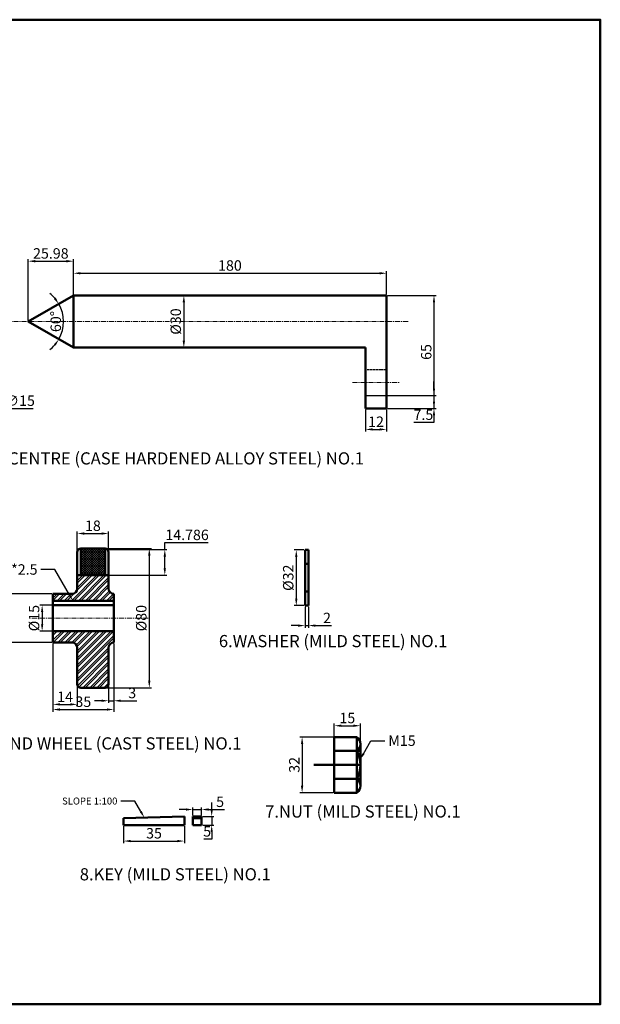
# Model space of a CAD drawing. Units: millimetres. Extents: x 177 to 1064, y 105 to 671.
# Tile 4 of 4: x 730 to 1064, y 105 to 671. Entities that reach past the tile are written whole.
import ezdxf
from ezdxf import colors
from ezdxf.entities.mleader import LeaderData, LeaderLine
from ezdxf.math import Vec2, Vec3

# ---------------------------------------------------------------- set-up
doc = ezdxf.new("R2010")
doc.units = ezdxf.units.MM
doc.header["$LTSCALE"] = 0.3
doc.linetypes.add('CENTER', pattern=[50.8, 31.75, -6.35, 6.35, -6.35])
doc.linetypes.add('HIDDEN', pattern=[9.525, 6.35, -3.175])
for name, color, linetype, lineweight in [('M-CNTR', 1, 'CENTER', 18), ('M-DIMS', 2, 'Continuous', 25), ('M-HATC', 8, 'Continuous', 18), ('M-HIDN', 6, 'HIDDEN', 25), ('M-OUTL', 7, 'Continuous', 50), ('M-TEXT', 3, 'Continuous', 25)]:
    doc.layers.add(name, color=color, linetype=linetype, lineweight=lineweight)
doc.styles.get("Standard").update_dxf_attribs({"font": 'arial.ttf'})
doc.dimstyles.new('ISO-25', dxfattribs={"dimtxt": 6, "dimasz": 4, "dimexe": 1.25, "dimexo": 0.625, "dimtad": 1, "dimtoh": 1, "dimtxsty": 'Standard', "dimcen": 2.5, "dimadec": 0, "dimazin": 0, "dimtfac": 1, "dimtmove": 0, "dimatfit": 3, "dimfxl": 1, "dimarcsym": 0})

# ---------------------------------------------------------------- blocks, each defined once
blk = doc.blocks.new('*D20')
at = {"layer": 'Defpoints', "color": 0, "ltscale": 0.3, "transparency": 16777216}
for p in [(940.65, 525.41), (760.65, 512.65), (940.65, 512.65)]:
    blk.add_point(p, dxfattribs=at)
at = {"layer": 'M-DIMS', "color": 0, "lineweight": -2, "ltscale": 0.3, "transparency": 16777216}
for p, q in [((760.65, 513.28), (760.65, 526.66)), ((940.65, 513.28), (940.65, 526.66)), ((764.65, 525.41), (936.65, 525.41))]:
    blk.add_line(p, q, dxfattribs=at)
at = {"layer": 'M-DIMS', "color": 0, "ltscale": 0.3, "transparency": 16777216}
for points in [[(764.65, 526.08), (764.65, 524.75), (760.65, 525.41)], [(936.65, 526.08), (936.65, 524.75), (940.65, 525.41)]]:
    blk.add_solid(points, dxfattribs=at)
at = {"layer": 'M-DIMS', "color": 0, "ltscale": 0.3, "transparency": 16777216, "insert": (850.65, 529.1), "char_height": 6, "attachment_point": 5}
blk.add_mtext('180', dxfattribs=at)
blk = doc.blocks.new('*D21')
at = {"layer": 'Defpoints', "color": 0, "ltscale": 0.3, "transparency": 16777216}
for p in [(821.8, 512.65), (821.8, 482.65), (824.15, 482.65)]:
    blk.add_point(p, dxfattribs=at)
at = {"layer": 'M-DIMS', "color": 0, "lineweight": -2, "ltscale": 0.3, "transparency": 16777216}
for p, q in [((822.42, 512.65), (825.4, 512.65)), ((824.15, 508.65), (824.15, 486.65)), ((822.42, 482.65), (825.4, 482.65))]:
    blk.add_line(p, q, dxfattribs=at)
at = {"layer": 'M-DIMS', "color": 0, "ltscale": 0.3, "transparency": 16777216}
for points in [[(823.48, 508.65), (824.82, 508.65), (824.15, 512.65)], [(823.48, 486.65), (824.82, 486.65), (824.15, 482.65)]]:
    blk.add_solid(points, dxfattribs=at)
at = {"layer": 'M-DIMS', "color": 0, "ltscale": 0.3, "transparency": 16777216, "insert": (820.29, 497.65), "char_height": 6, "attachment_point": 5, "rotation": 90}
blk.add_mtext('%%C30', dxfattribs=at)
blk = doc.blocks.new('*D22')
at = {"layer": 'Defpoints', "color": 0, "ltscale": 0.3, "transparency": 16777216}
for p in [(928.65, 447.65), (940.65, 447.65), (940.65, 435.63)]:
    blk.add_point(p, dxfattribs=at)
at = {"layer": 'M-DIMS', "color": 0, "lineweight": -2, "ltscale": 0.3, "transparency": 16777216}
for p, q in [((928.65, 447.03), (928.65, 434.38)), ((940.65, 447.03), (940.65, 434.38)), ((932.65, 435.63), (936.65, 435.63))]:
    blk.add_line(p, q, dxfattribs=at)
at = {"layer": 'M-DIMS', "color": 0, "ltscale": 0.3, "transparency": 16777216}
for points in [[(932.65, 436.3), (932.65, 434.97), (928.65, 435.63)], [(936.65, 436.3), (936.65, 434.97), (940.65, 435.63)]]:
    blk.add_solid(points, dxfattribs=at)
at = {"layer": 'M-DIMS', "color": 0, "ltscale": 0.3, "transparency": 16777216, "insert": (934.65, 439.27), "char_height": 6, "attachment_point": 5}
blk.add_mtext('12', dxfattribs=at)
blk = doc.blocks.new('*D25')
at = {"layer": 'Defpoints', "color": 0, "ltscale": 0.3, "transparency": 16777216}
for p in [(696.18, 467.24), (708.04, 458.06)]:
    blk.add_point(p, dxfattribs=at)
at = {"layer": 'M-DIMS', "color": 0, "lineweight": -2, "ltscale": 0.3, "transparency": 16777216}
for p, q in [((693.02, 469.69), (689.85, 472.14)), ((696.18, 467.24), (708.04, 458.06)), ((721.67, 447.51), (711.2, 455.61)), ((737.46, 447.51), (721.67, 447.51))]:
    blk.add_line(p, q, dxfattribs=at)
at = {"layer": 'M-DIMS', "color": 0, "ltscale": 0.3, "transparency": 16777216}
for points in [[(693.43, 470.22), (692.61, 469.16), (696.18, 467.24)], [(711.61, 456.14), (710.8, 455.08), (708.04, 458.06)]]:
    blk.add_solid(points, dxfattribs=at)
at = {"layer": 'M-DIMS', "color": 0, "ltscale": 0.3, "transparency": 16777216, "insert": (729.88, 451.37), "char_height": 6, "attachment_point": 5}
blk.add_mtext('∅15', dxfattribs=at)
blk = doc.blocks.new('*D26')
at = {"layer": 'Defpoints', "color": 0, "ltscale": 0.3, "transparency": 16777216}
for p in [(760.65, 512.65), (734.67, 497.65), (734.67, 497.65), (754.67, 494.12), (760.65, 482.65)]:
    blk.add_point(p, dxfattribs=at)
at = {"layer": 'M-DIMS', "color": 0, "lineweight": -2, "ltscale": 0.3, "transparency": 16777216}
for start, end in [(41.3018, 52.6036), (330, 30), (307.3964, 318.6982)]:
    blk.add_arc((734.67, 497.65), 20.31, start, end, dxfattribs=at)
at = {"layer": 'M-DIMS', "color": 0, "ltscale": 0.3, "transparency": 16777216}
for points in [[(750.47, 511.45), (749.39, 510.67), (752.26, 507.81)], [(749.39, 484.63), (750.47, 483.86), (752.26, 487.49)]]:
    blk.add_solid(points, dxfattribs=at)
at = {"layer": 'M-DIMS', "color": 0, "ltscale": 0.3, "transparency": 16777216, "insert": (751.29, 497.65), "char_height": 6, "attachment_point": 5, "rotation": 90}
blk.add_mtext('60°', dxfattribs=at)
blk = doc.blocks.new('*D27')
at = {"layer": 'Defpoints', "color": 0, "ltscale": 0.3, "transparency": 16777216}
for p in [(773.7, 367.13), (771.87, 287.13), (804.29, 287.13)]:
    blk.add_point(p, dxfattribs=at)
at = {"layer": 'M-DIMS', "color": 0, "lineweight": -2, "ltscale": 0.3, "transparency": 16777216}
for p, q in [((774.32, 367.13), (805.54, 367.13)), ((804.29, 363.13), (804.29, 291.13)), ((772.49, 287.13), (805.54, 287.13))]:
    blk.add_line(p, q, dxfattribs=at)
at = {"layer": 'M-DIMS', "color": 0, "ltscale": 0.3, "transparency": 16777216}
for points in [[(803.62, 363.13), (804.95, 363.13), (804.29, 367.13)], [(803.62, 291.13), (804.95, 291.13), (804.29, 287.13)]]:
    blk.add_solid(points, dxfattribs=at)
at = {"layer": 'M-DIMS', "color": 0, "ltscale": 0.3, "transparency": 16777216, "insert": (800.43, 327.13), "char_height": 6, "attachment_point": 5, "rotation": 90}
blk.add_mtext('%%C80', dxfattribs=at)
blk = doc.blocks.new('*D28')
at = {"layer": 'Defpoints', "color": 0, "ltscale": 0.3, "transparency": 16777216}
for p in [(780.87, 375.78), (762.87, 365.13), (780.87, 365.13)]:
    blk.add_point(p, dxfattribs=at)
at = {"layer": 'M-DIMS', "color": 0, "lineweight": -2, "ltscale": 0.3, "transparency": 16777216}
for p, q in [((762.87, 365.76), (762.87, 377.03)), ((766.87, 375.78), (776.87, 375.78)), ((780.87, 365.76), (780.87, 377.03))]:
    blk.add_line(p, q, dxfattribs=at)
at = {"layer": 'M-DIMS', "color": 0, "ltscale": 0.3, "transparency": 16777216}
for points in [[(766.87, 376.44), (766.87, 375.11), (762.87, 375.78)], [(776.87, 376.44), (776.87, 375.11), (780.87, 375.78)]]:
    blk.add_solid(points, dxfattribs=at)
at = {"layer": 'M-DIMS', "color": 0, "ltscale": 0.3, "transparency": 16777216, "insert": (771.87, 379.46), "char_height": 6, "attachment_point": 5}
blk.add_mtext('18', dxfattribs=at)
blk = doc.blocks.new('*D29')
at = {"layer": 'Defpoints', "color": 0, "ltscale": 0.3, "transparency": 16777216}
for p in [(748.87, 341.13), (720.48, 313.13), (748.87, 313.13)]:
    blk.add_point(p, dxfattribs=at)
at = {"layer": 'M-DIMS', "color": 0, "lineweight": -2, "ltscale": 0.3, "transparency": 16777216}
for p, q in [((748.24, 341.13), (719.23, 341.13)), ((720.48, 337.13), (720.48, 317.13)), ((748.24, 313.13), (719.23, 313.13))]:
    blk.add_line(p, q, dxfattribs=at)
at = {"layer": 'M-DIMS', "color": 0, "ltscale": 0.3, "transparency": 16777216}
for points in [[(719.81, 337.13), (721.14, 337.13), (720.48, 341.13)], [(719.81, 317.13), (721.14, 317.13), (720.48, 313.13)]]:
    blk.add_solid(points, dxfattribs=at)
at = {"layer": 'M-DIMS', "color": 0, "ltscale": 0.3, "transparency": 16777216, "insert": (716.62, 327.13), "char_height": 6, "attachment_point": 5, "rotation": 90}
blk.add_mtext('%%C28', dxfattribs=at)
blk = doc.blocks.new('*D30')
at = {"layer": 'Defpoints', "color": 0, "ltscale": 0.3, "transparency": 16777216}
for p in [(756.31, 334.63), (742.67, 319.63), (756.31, 319.63)]:
    blk.add_point(p, dxfattribs=at)
at = {"layer": 'M-DIMS', "color": 0, "lineweight": -2, "ltscale": 0.3, "transparency": 16777216}
for p, q in [((755.68, 334.63), (741.42, 334.63)), ((742.67, 330.63), (742.67, 323.63)), ((755.68, 319.63), (741.42, 319.63))]:
    blk.add_line(p, q, dxfattribs=at)
at = {"layer": 'M-DIMS', "color": 0, "ltscale": 0.3, "transparency": 16777216}
for points in [[(742.01, 330.63), (743.34, 330.63), (742.67, 334.63)], [(742.01, 323.63), (743.34, 323.63), (742.67, 319.63)]]:
    blk.add_solid(points, dxfattribs=at)
at = {"layer": 'M-DIMS', "color": 0, "ltscale": 0.3, "transparency": 16777216, "insert": (738.82, 327.13), "char_height": 6, "attachment_point": 5, "rotation": 90}
blk.add_mtext('%%C15', dxfattribs=at)
blk = doc.blocks.new('*D31')
at = {"layer": 'Defpoints', "color": 0, "ltscale": 0.3, "transparency": 16777216}
for p in [(748.87, 313.13), (783.87, 313.13), (783.87, 274.59)]:
    blk.add_point(p, dxfattribs=at)
at = {"layer": 'M-DIMS', "color": 0, "lineweight": -2, "ltscale": 0.3, "transparency": 16777216}
for p, q in [((748.87, 312.51), (748.87, 273.34)), ((783.87, 312.51), (783.87, 273.34)), ((752.87, 274.59), (779.87, 274.59))]:
    blk.add_line(p, q, dxfattribs=at)
at = {"layer": 'M-DIMS', "color": 0, "ltscale": 0.3, "transparency": 16777216}
for points in [[(752.87, 275.26), (752.87, 273.92), (748.87, 274.59)], [(779.87, 275.26), (779.87, 273.92), (783.87, 274.59)]]:
    blk.add_solid(points, dxfattribs=at)
at = {"layer": 'M-DIMS', "color": 0, "ltscale": 0.3, "transparency": 16777216, "insert": (766.37, 278.28), "char_height": 6, "attachment_point": 5}
blk.add_mtext('35', dxfattribs=at)
blk = doc.blocks.new('*D32')
at = {"layer": 'Defpoints', "color": 0, "ltscale": 0.3, "transparency": 16777216}
for p in [(780.87, 291.61), (783.87, 291.61), (783.87, 279.64)]:
    blk.add_point(p, dxfattribs=at)
at = {"layer": 'M-DIMS', "color": 0, "lineweight": -2, "ltscale": 0.3, "transparency": 16777216}
for p, q in [((780.87, 290.99), (780.87, 278.39)), ((783.87, 290.99), (783.87, 278.39)), ((776.87, 279.64), (772.87, 279.64)), ((780.87, 279.64), (783.87, 279.64)), ((787.87, 279.64), (797.05, 279.64))]:
    blk.add_line(p, q, dxfattribs=at)
at = {"layer": 'M-DIMS', "color": 0, "ltscale": 0.3, "transparency": 16777216}
for points in [[(776.87, 280.3), (776.87, 278.97), (780.87, 279.64)], [(787.87, 280.3), (787.87, 278.97), (783.87, 279.64)]]:
    blk.add_solid(points, dxfattribs=at)
at = {"layer": 'M-DIMS', "color": 0, "ltscale": 0.3, "transparency": 16777216, "insert": (794.46, 283.33), "char_height": 6, "attachment_point": 5}
blk.add_mtext('3', dxfattribs=at)
blk = doc.blocks.new('*D44')
at = {"layer": 'Defpoints', "color": 0, "ltscale": 0.3, "transparency": 16777216}
for p in [(893.84, 366.35), (888.79, 334.35), (893.84, 334.35)]:
    blk.add_point(p, dxfattribs=at)
at = {"layer": 'M-DIMS', "color": 0, "lineweight": -2, "ltscale": 0.3, "transparency": 16777216}
for p, q in [((893.22, 366.35), (887.54, 366.35)), ((888.79, 362.35), (888.79, 338.35)), ((893.22, 334.35), (887.54, 334.35))]:
    blk.add_line(p, q, dxfattribs=at)
at = {"layer": 'M-DIMS', "color": 0, "ltscale": 0.3, "transparency": 16777216}
for points in [[(888.13, 362.35), (889.46, 362.35), (888.79, 366.35)], [(888.13, 338.35), (889.46, 338.35), (888.79, 334.35)]]:
    blk.add_solid(points, dxfattribs=at)
at = {"layer": 'M-DIMS', "color": 0, "ltscale": 0.3, "transparency": 16777216, "insert": (884.94, 350.35), "char_height": 6, "attachment_point": 5, "rotation": 90}
blk.add_mtext('%%C32', dxfattribs=at)
blk = doc.blocks.new('*D45')
at = {"layer": 'Defpoints', "color": 0, "ltscale": 0.3, "transparency": 16777216}
for p in [(893.84, 334.35), (895.84, 334.35), (895.84, 322.84)]:
    blk.add_point(p, dxfattribs=at)
at = {"layer": 'M-DIMS', "color": 0, "lineweight": -2, "ltscale": 0.3, "transparency": 16777216}
for p, q in [((893.84, 333.72), (893.84, 321.59)), ((895.84, 333.72), (895.84, 321.59)), ((889.84, 322.84), (885.84, 322.84)), ((893.84, 322.84), (895.84, 322.84)), ((899.84, 322.84), (909.07, 322.84))]:
    blk.add_line(p, q, dxfattribs=at)
at = {"layer": 'M-DIMS', "color": 0, "ltscale": 0.3, "transparency": 16777216}
for points in [[(889.84, 323.5), (889.84, 322.17), (893.84, 322.84)], [(899.84, 323.5), (899.84, 322.17), (895.84, 322.84)]]:
    blk.add_solid(points, dxfattribs=at)
at = {"layer": 'M-DIMS', "color": 0, "ltscale": 0.3, "transparency": 16777216, "insert": (906.45, 326.47), "char_height": 6, "attachment_point": 5}
blk.add_mtext('2', dxfattribs=at)
blk = doc.blocks.new('*D46')
at = {"layer": 'Defpoints', "color": 0, "ltscale": 0.3, "transparency": 16777216}
for p in [(925.66, 265.27), (910.66, 250.76), (925.66, 250.76)]:
    blk.add_point(p, dxfattribs=at)
at = {"layer": 'M-DIMS', "color": 0, "lineweight": -2, "ltscale": 0.3, "transparency": 16777216}
for p, q in [((910.66, 251.38), (910.66, 266.52)), ((925.66, 251.38), (925.66, 266.52)), ((914.66, 265.27), (921.66, 265.27))]:
    blk.add_line(p, q, dxfattribs=at)
at = {"layer": 'M-DIMS', "color": 0, "ltscale": 0.3, "transparency": 16777216}
for points in [[(914.66, 265.93), (914.66, 264.6), (910.66, 265.27)], [(921.66, 265.93), (921.66, 264.6), (925.66, 265.27)]]:
    blk.add_solid(points, dxfattribs=at)
at = {"layer": 'M-DIMS', "color": 0, "ltscale": 0.3, "transparency": 16777216, "insert": (918.16, 268.95), "char_height": 6, "attachment_point": 5}
blk.add_mtext('15', dxfattribs=at)
blk = doc.blocks.new('*D47')
at = {"layer": 'Defpoints', "color": 0, "ltscale": 0.3, "transparency": 16777216}
for p in [(834.39, 217.09), (829.39, 213.1), (834.39, 213.1)]:
    blk.add_point(p, dxfattribs=at)
at = {"layer": 'M-DIMS', "color": 0, "lineweight": -2, "ltscale": 0.3, "transparency": 16777216}
for p, q in [((825.39, 217.09), (821.39, 217.09)), ((829.39, 213.73), (829.39, 218.34)), ((829.39, 217.09), (834.39, 217.09)), ((834.39, 213.73), (834.39, 218.34)), ((838.39, 217.09), (847.62, 217.09))]:
    blk.add_line(p, q, dxfattribs=at)
at = {"layer": 'M-DIMS', "color": 0, "ltscale": 0.3, "transparency": 16777216}
for points in [[(825.39, 217.76), (825.39, 216.43), (829.39, 217.09)], [(838.39, 217.76), (838.39, 216.43), (834.39, 217.09)]]:
    blk.add_solid(points, dxfattribs=at)
at = {"layer": 'M-DIMS', "color": 0, "ltscale": 0.3, "transparency": 16777216, "insert": (845, 220.77), "char_height": 6, "attachment_point": 5}
blk.add_mtext('5', dxfattribs=at)
blk = doc.blocks.new('*D48')
at = {"layer": 'Defpoints', "color": 0, "ltscale": 0.3, "transparency": 16777216}
for p in [(834.39, 213.1), (834.39, 208.1), (840.16, 208.1)]:
    blk.add_point(p, dxfattribs=at)
at = {"layer": 'M-DIMS', "color": 0, "lineweight": -2, "ltscale": 0.3, "transparency": 16777216}
for p, q in [((840.16, 217.1), (840.16, 221.1)), ((835.01, 213.1), (841.41, 213.1)), ((840.16, 213.1), (840.16, 208.1)), ((835.01, 208.1), (841.41, 208.1)), ((840.16, 204.1), (840.16, 200.1)), ((840.16, 200.1), (835.56, 200.1))]:
    blk.add_line(p, q, dxfattribs=at)
at = {"layer": 'M-DIMS', "color": 0, "ltscale": 0.3, "transparency": 16777216}
for points in [[(839.49, 217.1), (840.83, 217.1), (840.16, 213.1)], [(839.49, 204.1), (840.83, 204.1), (840.16, 208.1)]]:
    blk.add_solid(points, dxfattribs=at)
at = {"layer": 'M-DIMS', "color": 0, "ltscale": 0.3, "transparency": 16777216, "insert": (837.55, 203.78), "char_height": 6, "attachment_point": 5}
blk.add_mtext('5', dxfattribs=at)
blk = doc.blocks.new('*D49')
at = {"layer": 'Defpoints', "color": 0, "ltscale": 0.3, "transparency": 16777216}
for p in [(789.5, 208.1), (824.5, 208.1), (824.5, 198.97)]:
    blk.add_point(p, dxfattribs=at)
at = {"layer": 'M-DIMS', "color": 0, "lineweight": -2, "ltscale": 0.3, "transparency": 16777216}
for p, q in [((789.5, 207.48), (789.5, 197.72)), ((824.5, 207.48), (824.5, 197.72)), ((793.5, 198.97), (820.5, 198.97))]:
    blk.add_line(p, q, dxfattribs=at)
at = {"layer": 'M-DIMS', "color": 0, "ltscale": 0.3, "transparency": 16777216}
for points in [[(793.5, 199.63), (793.5, 198.3), (789.5, 198.97)], [(820.5, 199.63), (820.5, 198.3), (824.5, 198.97)]]:
    blk.add_solid(points, dxfattribs=at)
at = {"layer": 'M-DIMS', "color": 0, "ltscale": 0.3, "transparency": 16777216, "insert": (807, 202.66), "char_height": 6, "attachment_point": 5}
blk.add_mtext('35', dxfattribs=at)
blk = doc.blocks.new('*D61')
at = {"layer": 'Defpoints', "color": 0, "ltscale": 0.3, "transparency": 16777216}
for p in [(760.65, 532.34), (760.65, 512.65), (734.67, 497.65)]:
    blk.add_point(p, dxfattribs=at)
at = {"layer": 'M-DIMS', "color": 0, "lineweight": -2, "ltscale": 0.3, "transparency": 16777216}
for p, q in [((734.67, 498.28), (734.67, 533.59)), ((738.67, 532.34), (756.65, 532.34)), ((760.65, 513.28), (760.65, 533.59))]:
    blk.add_line(p, q, dxfattribs=at)
at = {"layer": 'M-DIMS', "color": 0, "ltscale": 0.3, "transparency": 16777216}
for points in [[(738.67, 533.01), (738.67, 531.67), (734.67, 532.34)], [(756.65, 533.01), (756.65, 531.67), (760.65, 532.34)]]:
    blk.add_solid(points, dxfattribs=at)
at = {"layer": 'M-DIMS', "color": 0, "ltscale": 0.3, "transparency": 16777216, "insert": (747.66, 536.03), "char_height": 6, "attachment_point": 5}
blk.add_mtext('25.98', dxfattribs=at)
blk = doc.blocks.new('*D62')
at = {"layer": 'Defpoints', "color": 0, "ltscale": 0.3, "transparency": 16777216}
for p in [(940.65, 512.65), (940.65, 447.65), (967.98, 447.65)]:
    blk.add_point(p, dxfattribs=at)
at = {"layer": 'M-DIMS', "color": 0, "lineweight": -2, "ltscale": 0.3, "transparency": 16777216}
for p, q in [((941.28, 512.65), (969.23, 512.65)), ((967.98, 508.65), (967.98, 451.65)), ((941.28, 447.65), (969.23, 447.65))]:
    blk.add_line(p, q, dxfattribs=at)
at = {"layer": 'M-DIMS', "color": 0, "ltscale": 0.3, "transparency": 16777216}
for points in [[(967.31, 508.65), (968.64, 508.65), (967.98, 512.65)], [(967.31, 451.65), (968.64, 451.65), (967.98, 447.65)]]:
    blk.add_solid(points, dxfattribs=at)
at = {"layer": 'M-DIMS', "color": 0, "ltscale": 0.3, "transparency": 16777216, "insert": (964.29, 480.15), "char_height": 6, "attachment_point": 5, "rotation": 90}
blk.add_mtext('65', dxfattribs=at)
blk = doc.blocks.new('*D63')
at = {"layer": 'Defpoints', "color": 0, "ltscale": 0.3, "transparency": 16777216}
for p in [(928.65, 455.15), (940.65, 447.65), (967.98, 447.65)]:
    blk.add_point(p, dxfattribs=at)
at = {"layer": 'M-DIMS', "color": 0, "lineweight": -2, "ltscale": 0.3, "transparency": 16777216}
for p, q in [((967.98, 459.15), (967.98, 463.15)), ((929.28, 455.15), (969.23, 455.15)), ((967.98, 455.15), (967.98, 447.65)), ((941.28, 447.65), (969.23, 447.65)), ((967.98, 443.65), (967.98, 439.65)), ((967.98, 439.65), (956.43, 439.65))]:
    blk.add_line(p, q, dxfattribs=at)
at = {"layer": 'M-DIMS', "color": 0, "ltscale": 0.3, "transparency": 16777216}
for points in [[(967.31, 459.15), (968.64, 459.15), (967.98, 455.15)], [(967.31, 443.65), (968.64, 443.65), (967.98, 447.65)]]:
    blk.add_solid(points, dxfattribs=at)
at = {"layer": 'M-DIMS', "color": 0, "ltscale": 0.3, "transparency": 16777216, "insert": (961.89, 443.33), "char_height": 6, "attachment_point": 5}
blk.add_mtext('7.5', dxfattribs=at)
blk = doc.blocks.new('*D64')
at = {"layer": 'Defpoints', "color": 0, "ltscale": 0.3, "transparency": 16777216}
for p in [(780.28, 366.55), (813.2, 366.55), (780.87, 351.76)]:
    blk.add_point(p, dxfattribs=at)
at = {"layer": 'M-DIMS', "color": 0, "lineweight": -2, "ltscale": 0.3, "transparency": 16777216}
for p, q in [((813.2, 366.55), (813.2, 370.55)), ((813.2, 370.55), (838.16, 370.55)), ((780.91, 366.55), (814.45, 366.55)), ((813.2, 355.76), (813.2, 362.55)), ((781.49, 351.76), (814.45, 351.76))]:
    blk.add_line(p, q, dxfattribs=at)
at = {"layer": 'M-DIMS', "color": 0, "ltscale": 0.3, "transparency": 16777216}
for points in [[(812.53, 362.55), (813.86, 362.55), (813.2, 366.55)], [(812.53, 355.76), (813.86, 355.76), (813.2, 351.76)]]:
    blk.add_solid(points, dxfattribs=at)
at = {"layer": 'M-DIMS', "color": 0, "ltscale": 0.3, "transparency": 16777216, "insert": (825.99, 374.23), "char_height": 6, "attachment_point": 5}
blk.add_mtext('14.786', dxfattribs=at)
blk = doc.blocks.new('*D65')
at = {"layer": 'Defpoints', "color": 0, "ltscale": 0.3, "transparency": 16777216}
for p in [(748.87, 313.13), (762.87, 310.13), (762.87, 277.53)]:
    blk.add_point(p, dxfattribs=at)
at = {"layer": 'M-DIMS', "color": 0, "lineweight": -2, "ltscale": 0.3, "transparency": 16777216}
for p, q in [((748.87, 312.51), (748.87, 276.28)), ((762.87, 309.51), (762.87, 276.28)), ((752.87, 277.53), (758.87, 277.53))]:
    blk.add_line(p, q, dxfattribs=at)
at = {"layer": 'M-DIMS', "color": 0, "ltscale": 0.3, "transparency": 16777216}
for points in [[(752.87, 278.2), (752.87, 276.87), (748.87, 277.53)], [(758.87, 278.2), (758.87, 276.87), (762.87, 277.53)]]:
    blk.add_solid(points, dxfattribs=at)
at = {"layer": 'M-DIMS', "color": 0, "ltscale": 0.3, "transparency": 16777216, "insert": (755.87, 281.17), "char_height": 6, "attachment_point": 5}
blk.add_mtext('14', dxfattribs=at)
blk = doc.blocks.new('*D67')
at = {"layer": 'Defpoints', "color": 0, "ltscale": 0.3, "transparency": 16777216}
for p in [(910.66, 258.76), (892.14, 226.76), (910.66, 226.76)]:
    blk.add_point(p, dxfattribs=at)
at = {"layer": 'M-DIMS', "color": 0, "lineweight": -2, "ltscale": 0.3, "transparency": 16777216}
for p, q in [((910.04, 258.76), (890.89, 258.76)), ((892.14, 254.76), (892.14, 230.76)), ((910.04, 226.76), (890.89, 226.76))]:
    blk.add_line(p, q, dxfattribs=at)
at = {"layer": 'M-DIMS', "color": 0, "ltscale": 0.3, "transparency": 16777216}
for points in [[(891.47, 254.76), (892.81, 254.76), (892.14, 258.76)], [(891.47, 230.76), (892.81, 230.76), (892.14, 226.76)]]:
    blk.add_solid(points, dxfattribs=at)
at = {"layer": 'M-DIMS', "color": 0, "ltscale": 0.3, "transparency": 16777216, "insert": (888.45, 242.76), "char_height": 6, "attachment_point": 5, "rotation": 90}
blk.add_mtext('32', dxfattribs=at)

msp = doc.modelspace()

# ---------------------------------------------------------------- hatches: boundary and pattern name
at = {"layer": 'M-HATC', "ltscale": 0.3}
h = msp.add_hatch(dxfattribs=at)
h.set_pattern_fill('ANSI37', color=256, scale=0.3)
h.set_pattern_definition([(45, (-544.7155, -110.339), (-0.6735192, 0.6735192), []), (135, (-544.7155, -110.339), (-0.6735192, -0.6735192), [])])
h.paths.add_polyline_path([(778.8685, 367.1319), (764.8685, 367.1319), (764.8685, 351.76), (778.8685, 351.76)])
h = msp.add_hatch(dxfattribs=at)
h.set_pattern_fill('ANSI32', color=256, scale=0.3)
h.set_pattern_definition([(45, (-544.7155, -110.339), (-2.0205576, 2.0205576), []), (45, (-543.3684, -110.339), (-2.0205576, 2.0205576), [])])
h.paths.add_polyline_path([(783.8685, 337.1319), (783.8685, 341.1319, -0.41421356), (780.8685, 344.1319), (780.8685, 351.76), (762.8685, 351.76), (762.8685, 344.1319, -0.41421356), (759.8685, 341.1319), (748.8685, 341.1319), (748.8685, 337.1319)])
h.paths.add_polyline_path([(780.8685, 310.1319, -0.41421356), (783.8685, 313.1319), (783.8685, 319.6319), (748.8685, 319.6319), (748.8685, 313.1319), (759.8685, 313.1319, -0.41421356), (762.8685, 310.1319), (762.8685, 289.1319, 0.41421356), (764.8685, 287.1319), (778.8685, 287.1319, 0.41421356), (780.8685, 289.1319)])

# ---------------------------------------------------------------- linework, layer by layer
at = {"layer": 'M-CNTR', "ltscale": 0.3}
for p, q in [((717.1114, 497.6506), (953.625, 497.6506)), ((921.1508, 462.6506), (948.3171, 462.6506)), ((736.7234, 327.1319), (803.5975, 327.1319))]:
    msp.add_line(p, q, dxfattribs=at)
at = {"layer": 'M-HIDN', "ltscale": 0.3}
for p, q in [((928.6524, 470.1506), (940.6524, 470.1506)), ((928.6524, 455.1506), (940.6524, 455.1506))]:
    msp.add_line(p, q, dxfattribs=at)
at = {"layer": 'M-OUTL', "ltscale": 0.3}
for p, q in [((760.6524, 512.6506), (734.6716, 497.6506)), ((760.6524, 482.6506), (760.6524, 512.6506)), ((760.6524, 512.6506), (940.6524, 512.6506)), ((940.6524, 512.6506), (940.6524, 447.6506)), ((760.6524, 482.6506), (734.6716, 497.6506)), ((928.6524, 482.6506), (760.6524, 482.6506)), ((928.6524, 447.6506), (928.6524, 482.6506)), ((928.6524, 447.6506), (940.6524, 447.6506)), ((762.8685, 344.1319), (762.8685, 365.1319)), ((764.8685, 367.1319), (778.8685, 367.1319)), ((764.8685, 351.76), (764.8685, 367.1319)), ((778.8685, 351.76), (778.8685, 367.1319)), ((780.8685, 344.1319), (780.8685, 365.1319)), ((893.8418, 366.3492), (895.8418, 366.3492)), ((893.8418, 334.3492), (893.8418, 366.3492)), ((895.8418, 366.3492), (895.8418, 334.3492)), ((895.8418, 358.3492), (893.8418, 358.3492)), ((762.8685, 351.76), (780.8685, 351.76)), ((748.8685, 341.1319), (759.8685, 341.1319)), ((748.8685, 327.1319), (748.8685, 341.1319)), ((783.8685, 341.1319), (783.8685, 341.1319)), ((783.8685, 327.1319), (783.8685, 341.1319)), ((895.8418, 342.3492), (893.8418, 342.3492)), ((748.8685, 337.1319), (783.8685, 337.1319)), ((748.8685, 334.6319), (783.8685, 334.6319)), ((783.8685, 334.6319), (783.8685, 327.1319)), ((895.8418, 334.3492), (893.8418, 334.3492)), ((748.8685, 327.1319), (748.8685, 313.1319)), ((783.8685, 319.6319), (783.8685, 327.1319)), ((783.8685, 327.1319), (783.8685, 313.1319)), ((748.8685, 319.6319), (783.8685, 319.6319)), ((748.8685, 313.1319), (759.8685, 313.1319)), ((783.8685, 313.1319), (783.8685, 313.1319)), ((762.8685, 310.1319), (762.8685, 289.1319)), ((780.8685, 310.1319), (780.8685, 289.1319)), ((764.8685, 287.1319), (778.8685, 287.1319)), ((910.6638, 258.7587), (910.6638, 226.7587)), ((923.6638, 258.7587), (910.6638, 258.7587)), ((923.6638, 226.7587), (923.6638, 258.7587)), ((925.6638, 230.3178), (925.6638, 255.2952)), ((910.6638, 250.7587), (925.6638, 250.7587)), ((898.8913, 242.7587), (925.6638, 242.7587)), ((910.6638, 234.7587), (925.6638, 234.7587)), ((910.6638, 226.7587), (923.6638, 226.7587)), ((789.5025, 212.1009), (824.5025, 213.1009)), ((789.5025, 208.1009), (789.5025, 212.1009)), ((824.5025, 208.1009), (824.5025, 213.1009)), ((829.3895, 213.1009), (829.3895, 208.1009)), ((834.3895, 213.1009), (829.3895, 213.1009)), ((834.3895, 212.1009), (829.3895, 212.1009)), ((834.3895, 208.1009), (834.3895, 213.1009)), ((789.5025, 208.1009), (824.5025, 208.1009)), ((829.3895, 208.1009), (834.3895, 208.1009))]:
    msp.add_line(p, q, dxfattribs=at)
msp.add_lwpolyline([(176.7558, 671.1865), (1063.6064, 671.1865), (1063.6064, 105.1095), (176.7558, 105.1095)], close=True, dxfattribs=at)
for centre, radius, start, end in [((764.8685, 365.1319), 2, 90, 180), ((778.8685, 365.1319), 2, 0, 90), ((759.8685, 344.1319), 3, 270, 0), ((783.8685, 344.1319), 3, 180, 270), ((759.8685, 310.1319), 3, 0, 90), ((783.8685, 310.1319), 3, 90, 180), ((764.8685, 289.1319), 2, 180, 270), ((778.8685, 289.1319), 2, 270, 0), ((920.7358, 254.7587), 4.9571, 306.204359, 53.795641), ((908.6638, 242.7587), 17, 331.927513, 28.072487), ((920.7124, 230.7587), 4.971, 306.421873, 53.578127)]:
    msp.add_arc(centre, radius, start, end, dxfattribs=at)

# ---------------------------------------------------------------- texts
at = {"layer": 'M-TEXT', "ltscale": 0.3, "char_height": 7, "attachment_point": 1}
for s, width, insert in [('\\pxqc;2. CENTRE (CASE HARDENED ALLOY STEEL) NO.1', 275.896457, (682.4091, 422.4621)), ('\\pxqc;6.WASHER (MILD STEEL) NO.1', 180.935096, (819.541, 317.4292)), ('\\pxqc;3.HAND WHEEL (CAST STEEL) NO.1', 180.935096, (689.8312, 258.6014)), ('\\pxqc;7.NUT (MILD STEEL) NO.1', 180.935096, (836.6256, 219.468)), ('\\pxqc;8.KEY (MILD STEEL) NO.1', 180.935096, (728.7463, 183.3548))]:
    msp.add_mtext_dynamic_manual_height_columns(s, width=width, gutter_width=12.5, heights=[0], dxfattribs=dict(at, insert=insert))

# ---------------------------------------------------------------- dimensions: what is measured, and where the dimension line sits
at = {"layer": 'M-DIMS', "ltscale": 0.3}
for base, p1, p2, override, picture, middle in [((760.6524, 532.3395), (734.6716, 497.6506), (760.6524, 512.6506), {"dimdec": 2, "dimlfac": 1, "dimrnd": 0, "dimzin": 0, "dimdsep": 46, "dimlunit": 2}, '*D61', (747.662, 536.028)), ((940.6524, 525.4128), (760.6524, 512.6506), (940.6524, 512.6506), {"dimclrd": 0, "dimclre": 0, "dimclrt": 0}, '*D20', (850.6524, 529.1012)), ((940.6524, 435.6328), (928.6524, 447.6506), (940.6524, 447.6506), {"dimclrd": 0, "dimclre": 0, "dimclrt": 0}, '*D22', (934.6524, 439.2701)), ((780.8685, 375.7759), (762.8685, 365.1319), (780.8685, 365.1319), {"dimclrd": 0, "dimclre": 0, "dimclrt": 0}, '*D28', (771.8685, 379.4644)), ((895.8418, 322.8377), (893.8418, 334.3492), (895.8418, 334.3492), {"dimclrd": 0, "dimclre": 0, "dimclrt": 0}, '*D45', (906.4538, 326.4749)), ((783.8685, 274.591), (748.8685, 313.1319), (783.8685, 313.1319), {"dimclrd": 0, "dimclre": 0, "dimclrt": 0}, '*D31', (766.3685, 278.2815)), ((762.8685, 277.5319), (748.8685, 313.1319), (762.8685, 310.1319), {"dimdec": 0, "dimlfac": 1, "dimrnd": 0, "dimzin": 0, "dimdsep": 46, "dimlunit": 2}, '*D65', (755.8685, 281.1692)), ((783.8685, 279.6351), (780.8685, 291.6147), (783.8685, 291.6147), {"dimclrd": 0, "dimclre": 0, "dimclrt": 0}, '*D32', (794.458, 283.3256)), ((925.6638, 265.2659), (910.6638, 250.7587), (925.6638, 250.7587), {"dimclrd": 0, "dimclre": 0, "dimclrt": 0}, '*D46', (918.1638, 268.9543)), ((834.3895, 217.0945), (829.3895, 213.1009), (834.3895, 213.1009), {"dimclrd": 0, "dimclre": 0, "dimclrt": 0}, '*D47', (845.0036, 220.7707))]:
    dim = msp.add_linear_dim(base=base, p1=p1, p2=p2, dimstyle='ISO-25', override=override, dxfattribs=at)
    dim.commit()
    dim.dimension.update_dxf_attribs({"geometry": picture, "text_midpoint": middle})
dim = msp.add_angular_dim_2l(base=(754.6744, 494.1235), line1=((760.6524, 482.6506), (734.6716, 497.6506)), line2=((760.6524, 512.6506), (734.6716, 497.6506)), dimstyle='ISO-25', override={"dimclrd": 0, "dimclre": 0, "dimclrt": 0}, dxfattribs=at)
dim.commit()
dim.dimension.update_dxf_attribs({"geometry": '*D26', "text_midpoint": (751.2945, 497.6506)})
for base, p1, p2, picture, middle in [((824.1492, 482.6506), (821.7958, 512.6506), (821.7958, 482.6506), '*D21', (820.293, 497.6506)), ((804.2869, 287.1319), (773.6999, 367.1319), (771.8685, 287.1319), '*D27', (800.4307, 327.1319)), ((888.7929, 334.3492), (893.8418, 366.3492), (893.8418, 334.3492), '*D44', (884.9367, 350.3492)), ((720.4777, 313.1319), (748.8685, 341.1319), (748.8685, 313.1319), '*D29', (716.6214, 327.1319))]:
    dim = msp.add_linear_dim(base=base, p1=p1, p2=p2, angle=90, text='%%C<>', dimstyle='ISO-25', override={"dimclrd": 0, "dimclre": 0, "dimclrt": 0}, dxfattribs=at)
    dim.commit()
    dim.dimension.update_dxf_attribs({"geometry": picture, "text_midpoint": middle})
for base, p1, p2, override, picture, middle in [((967.975, 447.6506), (940.6524, 512.6506), (940.6524, 447.6506), {"dimdec": 0, "dimlfac": 1, "dimrnd": 0, "dimzin": 0, "dimdsep": 46, "dimlunit": 2}, '*D62', (964.2866, 480.1506)), ((967.975, 447.6506), (928.6524, 455.1506), (940.6524, 447.6506), {"dimdec": 1, "dimlfac": 1, "dimrnd": 0, "dimzin": 0, "dimdsep": 46, "dimlunit": 2}, '*D63', (961.8903, 443.3267)), ((813.1975, 366.5461), (780.8685, 351.76), (780.2827, 366.5461), {"dimdec": 3, "dimlfac": 1, "dimrnd": 0, "dimzin": 0, "dimdsep": 46, "dimlunit": 2}, '*D64', (825.9924, 374.2345)), ((892.1413, 226.7587), (910.6638, 258.7587), (910.6638, 226.7587), {"dimdec": 0, "dimlfac": 1, "dimrnd": 0, "dimzin": 0, "dimdsep": 46, "dimlunit": 2}, '*D67', (888.4509, 242.7587)), ((840.1596, 208.1009), (834.3895, 213.1009), (834.3895, 208.1009), {"dimclrd": 0, "dimclre": 0, "dimclrt": 0}, '*D48', (837.5455, 203.7771))]:
    dim = msp.add_linear_dim(base=base, p1=p1, p2=p2, angle=90, dimstyle='ISO-25', override=override, dxfattribs=at)
    dim.commit()
    dim.dimension.update_dxf_attribs({"geometry": picture, "text_midpoint": middle})
dim = msp.add_diameter_dim_2p(p1=(696.1809, 467.2417), p2=(708.042, 458.0594), dimstyle='ISO-25', override={"dimclrd": 0, "dimclre": 0, "dimclrt": 0}, dxfattribs=at)
dim.commit()
dim.dimension.update_dxf_attribs({"geometry": '*D25', "text_midpoint": (729.8751, 447.5122), "dimtype": 163})
dim = msp.add_linear_dim(base=(742.6749, 319.6319), p1=(756.3076, 334.6319), p2=(756.3076, 319.6319), angle=90, text='%%C<>', dimstyle='ISO-25', override={"dimclrd": 0, "dimclre": 0, "dimclrt": 0}, dxfattribs=at)
dim.commit()
dim.dimension.update_dxf_attribs({"geometry": '*D30', "text_midpoint": (742.6749, 327.1319), "dimtype": 160})
dim = msp.add_linear_dim(base=(824.5025, 198.9656), p1=(789.5025, 208.1009), p2=(824.5025, 208.1009), dimstyle='ISO-25', override={"dimclrd": 0, "dimclre": 0, "dimclrt": 0}, dxfattribs=at)
dim.commit()
dim.dimension.update_dxf_attribs({"geometry": '*D49', "text_midpoint": (807.0025, 198.9656), "dimtype": 160})

# ---------------------------------------------------------------- leaders
ml = msp.add_multileader_mtext('Standard', dxfattribs=at)
ml.set_content('KEY WAY 5*2.5', color=256)
ml.set_leader_properties()
ml.build(insert=Vec2(0, 0))
ctx = ml.context
ctx.base_point, ctx.char_height, ctx.plane_origin = Vec3(678.8604, 355.0496), 6, Vec3(760.3538, 337.1319)
ctx.text_align_type = 2
notes = []
notes.append((ctx, [(0, (1, 1, 0), (750.0091, 355.0496), (-1, 0), 8, [(0, [(760.3538, 337.1319)], 0, [])])]))
ctx.mtext.insert, ctx.mtext.alignment, ctx.mtext.flow_direction = Vec3(740.0091, 358.1007), 3, 5
ml = msp.add_multileader_mtext('Standard', dxfattribs=at)
ml.set_content('M15', color=256)
ml.set_leader_properties()
ml.build(insert=Vec2(0, 0))
ctx = ml.context
ctx.base_point, ctx.char_height, ctx.plane_origin = Vec3(939.7163, 256.629), 6, Vec3(925.4072, 245.7013)
notes.append((ctx, [(0, (1, 1, 0), (931.7163, 256.629), (1, 0), 8, [(0, [(925.4072, 245.7013)], 0, [])])]))
ctx.mtext.insert, ctx.mtext.flow_direction = Vec3(941.7163, 259.6801), 5
ml = msp.add_multileader_mtext('Standard', dxfattribs=at)
ml.set_content('SLOPE 1:100', color=256)
ml.set_leader_properties()
ml.build(insert=Vec2(0, 0))
ctx = ml.context
ctx.base_point, ctx.plane_origin = Vec3(750.2879, 221.9409), Vec3(801.4259, 212.4416)
ctx.text_align_type = 2
notes.append((ctx, [(0, (1, 1, 0), (795.9414, 221.9409), (-1, 0), 8, [(0, [(801.4259, 212.4416)], 0, [])])]))
ctx.mtext.insert, ctx.mtext.alignment, ctx.mtext.flow_direction = Vec3(785.9414, 223.9751), 3, 5
for ctx, leaders in notes:
    for number, flags, end, landing, length, lines in leaders:
        leader = LeaderData()
        leader.index, (leader.has_last_leader_line, leader.has_dogleg_vector, leader.attachment_direction) = number, flags
        leader.last_leader_point, leader.dogleg_vector, leader.dogleg_length = Vec3(end), Vec3(landing), length
        for number, points, colour, breaks in lines:
            line = LeaderLine()
            line.index, line.vertices, line.color, line.breaks = number, Vec3.list(points), colors.encode_raw_color(colour), breaks
            leader.lines.append(line)
        ctx.leaders.append(leader)

doc.saveas('drawing.dxf')
